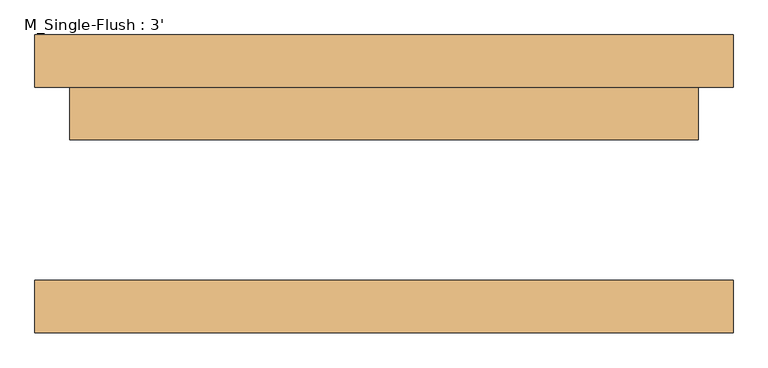
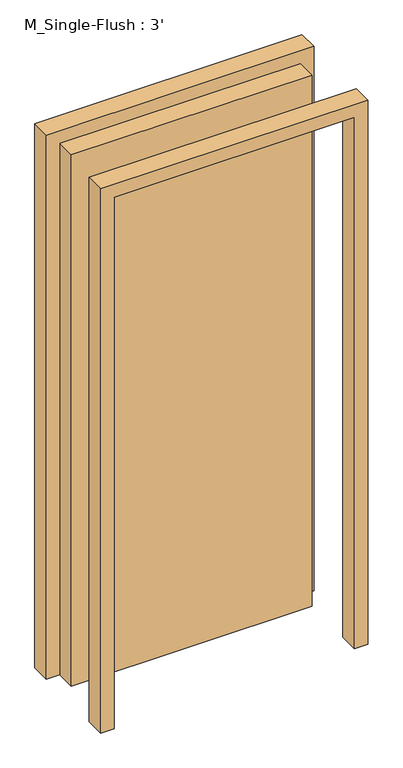
"""IFC4 building model written with IfcOpenShell, lengths in millimetres: door geometry, M_Single-Flush : 3'."""

from ifc_helpers import new_model, si_unit, frame, origin, origin_with_axes, place, context, project, spatial, polyline, outline, extrude, source, transform, mapped, element, save


def m_single_flush_3_17564fc7(model_context):
    return source(origin(), model_context, "Body", "SweptSolid", [
        extrude(outline(polyline([(2184.4, -508.0), (0.0, -508.0), (0.0, -457.2), (2133.6, -457.2), (2133.6, 457.2), (0.0, 457.2), (0.0, 508.0), (2184.4, 508.0), (2184.4, -508.0)])), frame((0.0, 140.4, 0.0), z_axis=(0.0, 1.0, 0.0), x_axis=(0.0, 0.0, 1.0)), (0.0, 0.0, 1.0), 76.2),
        extrude(outline(polyline([(2184.4, 508.0), (2184.4, -508.0), (0.0, -508.0), (0.0, -457.2), (2133.6, -457.2), (2133.6, 457.2), (0.0, 457.2), (0.0, 508.0), (2184.4, 508.0)])), frame((0.0, -216.6, 0.0), z_axis=(0.0, 1.0, 0.0), x_axis=(0.0, 0.0, 1.0)), (0.0, 0.0, 1.0), 76.2),
        extrude(outline(polyline([(457.2, 64.2), (-457.2, 64.2), (-457.2, 140.4), (457.2, 140.4), (457.2, 64.2)])), origin_with_axes(), (0.0, 0.0, 1.0), 2133.6),
    ])


if __name__ == "__main__":
    model = new_model("IFC4")
    model_context = context("Model", 3, world=origin())
    ifc_project = project(units=[si_unit("LENGTHUNIT", "METRE", prefix="MILLI")], contexts=[model_context])
    site = spatial("IfcSite", under=ifc_project)
    building = spatial("IfcBuilding", under=site)
    placement = place(None, origin())
    m_single_flush_3_shape = m_single_flush_3_17564fc7(model_context)
    element("IfcDoor", 1, ObjectType="M_Single-Flush : 3'", at=placement, inside=building, context=model_context, shape_type="MappedRepresentation", body=[
        mapped(m_single_flush_3_shape, transform((0.0, 0.0, 0.0), x_axis=(1.0, 0.0, 0.0), y_axis=(0.0, 1.0, 0.0), z_axis=(0.0, 0.0, 1.0))),
    ])
    save(model, "model.ifc")

# Revit data of these elements
# Type "M_Single-Flush : 3'"
#   Type Mark = "23"
#   Thickness = 0' - 3"
#   Height = 7' - 0"
#   Trim Projection Ext = 0' - 3"
#   Trim Projection Int = 0' - 3"
#   Trim Width = 0' - 2"
#   Width = 3' - 0"
#   Wall Closure = 2
#   Door Material = Door - Panel
#   Frame Material = Door - Panel
#   Function = (empty or 0)
# Element 1 (IfcDoor, "M_Single-Flush : 3'")
#   Materials on its faces: "Door - Panel"
# Materials
#   "Door - Panel": class "Wood", colour RGB 114 82 51, transparency 0
